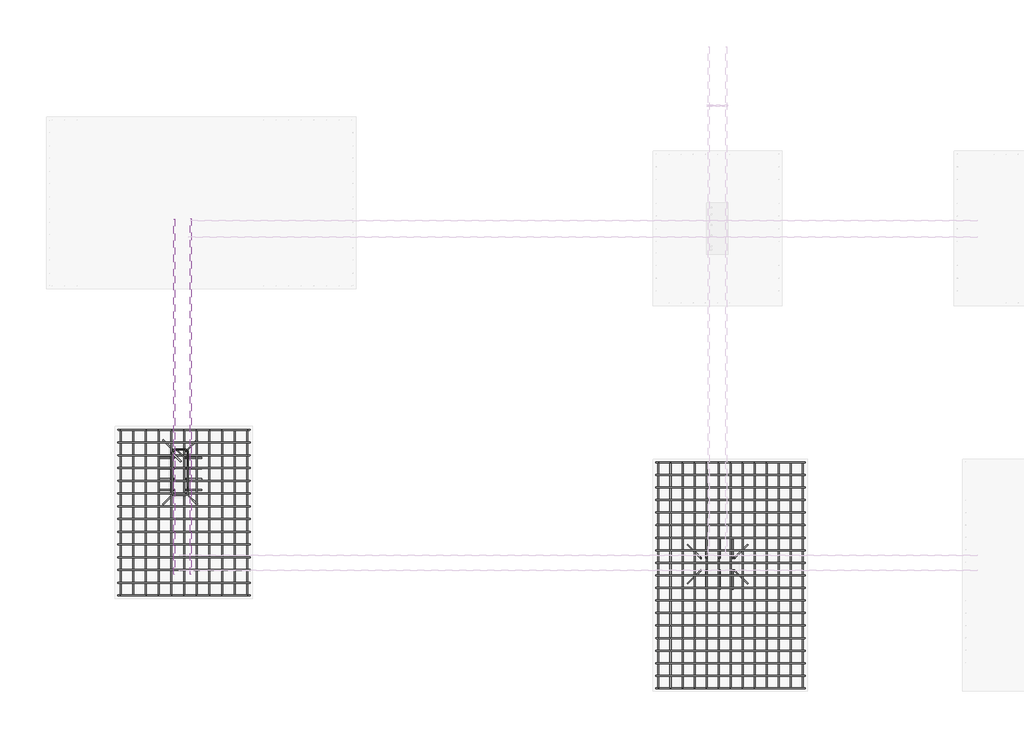
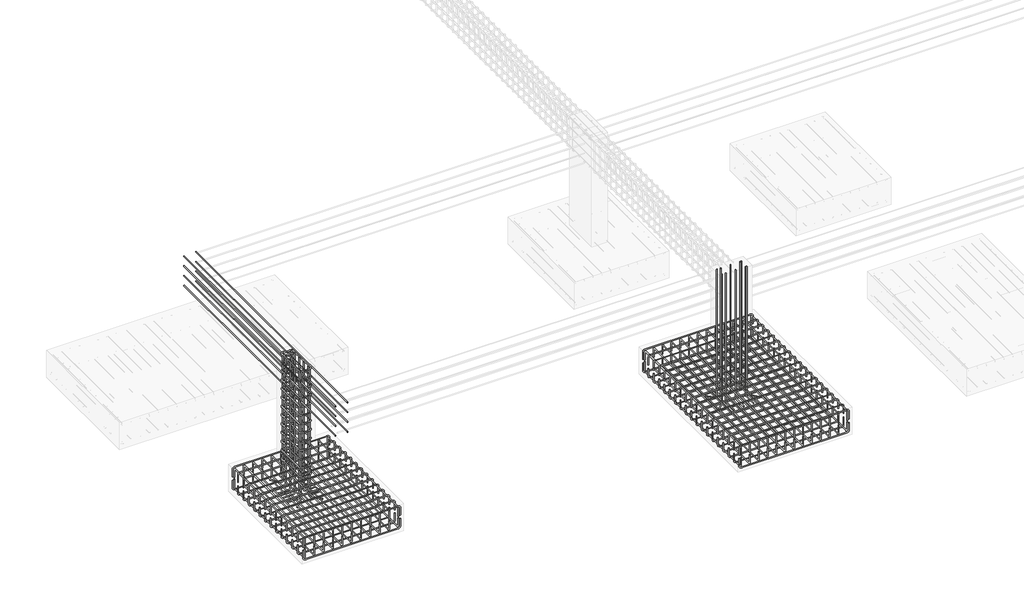
# One storey, part 2 of 16: 23 reinforcing bars.
"""IFC4 building model written with IfcOpenShell, lengths in millimetres."""

from ifc_helpers import new_model, si_unit, point, frame, origin, place, context, project, spatial, polyline, circle_curve, trimmed, segment, composite_curve, source, transform, mapped, element, save
from ifc_brep_helpers import swept_disk

model = new_model("IFC4")

# Units and contexts
model_context = context("Model", 3, world=origin())
ifc_project = project(units=[si_unit("LENGTHUNIT", "METRE", prefix="MILLI")], contexts=[model_context])

# Site, building, storey
site = spatial("IfcSite", under=ifc_project)
building = spatial("IfcBuilding", under=site)
storey = spatial("IfcBuildingStorey", under=building, Elevation=-1828.8)

# Reinforcing bars
placement = place(None, origin())
reinforcing_bar_shape = source(origin(), model_context, "Body", "SolidModel", [
    swept_disk(composite_curve([segment(polyline([(-7914.2725801, -5094.4085501, -2088.8), (-7914.2725801, -5094.4085501, -2212.8)]), True, "CONTINUOUS"), segment(trimmed(circle_curve(frame((-7944.2725801, -5094.4085501, -2212.8), z_axis=(0.0, 1.0, 0.0), x_axis=(30.0, 0.0, 0.0)), 30.0), [point((-7914.2725801, -5094.4085501, -2212.8))], [point((-7944.2725801, -5094.4085501, -2242.8))], True, "CARTESIAN"), True, "CONTINUOUS"), segment(polyline([(-7944.2725801, -5094.4085501, -2242.8), (-9612.2725801, -5094.4085501, -2242.8)]), True, "CONTINUOUS"), segment(trimmed(circle_curve(frame((-9612.2725801, -5094.4085501, -2212.8), z_axis=(0.0, 1.0, 0.0), x_axis=(0.0, 0.0, -30.0)), 30.0), [point((-9612.2725801, -5094.4085501, -2242.8))], [point((-9642.2725801, -5094.4085501, -2212.8))], True, "CARTESIAN"), True, "CONTINUOUS"), segment(polyline([(-9642.2725801, -5094.4085501, -2212.8), (-9642.2725801, -5094.4085501, -2088.8)]), True, "CONTINUOUS")], self_intersect=False), 6.0),
])
element("IfcReinforcingBar", 1, at=placement, inside=storey, context=model_context, shape_type="MappedRepresentation", body=[
    mapped(reinforcing_bar_shape, transform((0.0, 0.0, 0.0), x_axis=(1.0, 0.0, 0.0), y_axis=(0.0, 1.0, 0.0), z_axis=(0.0, 0.0, 1.0))),
    mapped(reinforcing_bar_shape, transform((0.0, -146.0, 0.0), x_axis=(1.0, 0.0, 0.0), y_axis=(0.0, 1.0, 0.0), z_axis=(0.0, 0.0, 1.0))),
    mapped(reinforcing_bar_shape, transform((0.0, -292.0, 0.0), x_axis=(1.0, 0.0, 0.0), y_axis=(0.0, 1.0, 0.0), z_axis=(0.0, 0.0, 1.0))),
    mapped(reinforcing_bar_shape, transform((0.0, -438.0, 0.0), x_axis=(1.0, 0.0, 0.0), y_axis=(0.0, 1.0, 0.0), z_axis=(0.0, 0.0, 1.0))),
    mapped(reinforcing_bar_shape, transform((0.0, -584.0, 0.0), x_axis=(1.0, 0.0, 0.0), y_axis=(0.0, 1.0, 0.0), z_axis=(0.0, 0.0, 1.0))),
    mapped(reinforcing_bar_shape, transform((0.0, -730.0, 0.0), x_axis=(1.0, 0.0, 0.0), y_axis=(0.0, 1.0, 0.0), z_axis=(0.0, 0.0, 1.0))),
    mapped(reinforcing_bar_shape, transform((0.0, -876.0, 0.0), x_axis=(1.0, 0.0, 0.0), y_axis=(0.0, 1.0, 0.0), z_axis=(0.0, 0.0, 1.0))),
    mapped(reinforcing_bar_shape, transform((0.0, -1022.0, 0.0), x_axis=(1.0, 0.0, 0.0), y_axis=(0.0, 1.0, 0.0), z_axis=(0.0, 0.0, 1.0))),
    mapped(reinforcing_bar_shape, transform((0.0, -1168.0, 0.0), x_axis=(1.0, 0.0, 0.0), y_axis=(0.0, 1.0, 0.0), z_axis=(0.0, 0.0, 1.0))),
    mapped(reinforcing_bar_shape, transform((0.0, -1314.0, 0.0), x_axis=(1.0, 0.0, 0.0), y_axis=(0.0, 1.0, 0.0), z_axis=(0.0, 0.0, 1.0))),
    mapped(reinforcing_bar_shape, transform((0.0, -1460.0, 0.0), x_axis=(1.0, 0.0, 0.0), y_axis=(0.0, 1.0, 0.0), z_axis=(0.0, 0.0, 1.0))),
    mapped(reinforcing_bar_shape, transform((0.0, -1606.0, 0.0), x_axis=(1.0, 0.0, 0.0), y_axis=(0.0, 1.0, 0.0), z_axis=(0.0, 0.0, 1.0))),
    mapped(reinforcing_bar_shape, transform((0.0, -1752.0, 0.0), x_axis=(1.0, 0.0, 0.0), y_axis=(0.0, 1.0, 0.0), z_axis=(0.0, 0.0, 1.0))),
    mapped(reinforcing_bar_shape, transform((0.0, -1898.0, 0.0), x_axis=(1.0, 0.0, 0.0), y_axis=(0.0, 1.0, 0.0), z_axis=(0.0, 0.0, 1.0))),
    mapped(reinforcing_bar_shape, transform((0.0, -2044.0, 0.0), x_axis=(1.0, 0.0, 0.0), y_axis=(0.0, 1.0, 0.0), z_axis=(0.0, 0.0, 1.0))),
    mapped(reinforcing_bar_shape, transform((0.0, -2190.0, 0.0), x_axis=(1.0, 0.0, 0.0), y_axis=(0.0, 1.0, 0.0), z_axis=(0.0, 0.0, 1.0))),
    mapped(reinforcing_bar_shape, transform((0.0, -2336.0, 0.0), x_axis=(1.0, 0.0, 0.0), y_axis=(0.0, 1.0, 0.0), z_axis=(0.0, 0.0, 1.0))),
    mapped(reinforcing_bar_shape, transform((0.0, -2482.0, 0.0), x_axis=(1.0, 0.0, 0.0), y_axis=(0.0, 1.0, 0.0), z_axis=(0.0, 0.0, 1.0))),
    mapped(reinforcing_bar_shape, transform((0.0, -2628.0, 0.0), x_axis=(1.0, 0.0, 0.0), y_axis=(0.0, 1.0, 0.0), z_axis=(0.0, 0.0, 1.0))),
])
reinforcing_bar_2_shape = source(origin(), model_context, "Body", "SolidModel", [
    swept_disk(composite_curve([segment(polyline([(-9642.2725801, -5094.4085501, -2024.671783), (-9642.2725801, -5094.4085501, -1900.671783)]), True, "CONTINUOUS"), segment(trimmed(circle_curve(frame((-9612.2725801, -5094.4085501, -1900.671783), z_axis=(0.0, 1.0, 0.0), x_axis=(-30.0, 0.0, 0.0)), 30.0), [point((-9642.2725801, -5094.4085501, -1900.671783))], [point((-9612.2725801, -5094.4085501, -1870.671783))], True, "CARTESIAN"), True, "CONTINUOUS"), segment(polyline([(-9612.2725801, -5094.4085501, -1870.671783), (-7944.2725801, -5094.4085501, -1870.671783)]), True, "CONTINUOUS"), segment(trimmed(circle_curve(frame((-7944.2725801, -5094.4085501, -1900.671783), z_axis=(0.0, 1.0, 0.0), x_axis=(0.0, 0.0, 30.0)), 30.0), [point((-7944.2725801, -5094.4085501, -1870.671783))], [point((-7914.2725801, -5094.4085501, -1900.671783))], True, "CARTESIAN"), True, "CONTINUOUS"), segment(polyline([(-7914.2725801, -5094.4085501, -1900.671783), (-7914.2725801, -5094.4085501, -2024.671783)]), True, "CONTINUOUS")], self_intersect=False), 6.0),
])
element("IfcReinforcingBar", 2, at=placement, inside=storey, context=model_context, shape_type="MappedRepresentation", body=[
    mapped(reinforcing_bar_2_shape, transform((0.0, 0.0, 0.0), x_axis=(1.0, 0.0, 0.0), y_axis=(0.0, 1.0, 0.0), z_axis=(0.0, 0.0, 1.0))),
    mapped(reinforcing_bar_2_shape, transform((0.0, -146.0, 0.0), x_axis=(1.0, 0.0, 0.0), y_axis=(0.0, 1.0, 0.0), z_axis=(0.0, 0.0, 1.0))),
    mapped(reinforcing_bar_2_shape, transform((0.0, -292.0, 0.0), x_axis=(1.0, 0.0, 0.0), y_axis=(0.0, 1.0, 0.0), z_axis=(0.0, 0.0, 1.0))),
    mapped(reinforcing_bar_2_shape, transform((0.0, -438.0, 0.0), x_axis=(1.0, 0.0, 0.0), y_axis=(0.0, 1.0, 0.0), z_axis=(0.0, 0.0, 1.0))),
    mapped(reinforcing_bar_2_shape, transform((0.0, -584.0, 0.0), x_axis=(1.0, 0.0, 0.0), y_axis=(0.0, 1.0, 0.0), z_axis=(0.0, 0.0, 1.0))),
    mapped(reinforcing_bar_2_shape, transform((0.0, -730.0, 0.0), x_axis=(1.0, 0.0, 0.0), y_axis=(0.0, 1.0, 0.0), z_axis=(0.0, 0.0, 1.0))),
    mapped(reinforcing_bar_2_shape, transform((0.0, -876.0, 0.0), x_axis=(1.0, 0.0, 0.0), y_axis=(0.0, 1.0, 0.0), z_axis=(0.0, 0.0, 1.0))),
    mapped(reinforcing_bar_2_shape, transform((0.0, -1022.0, 0.0), x_axis=(1.0, 0.0, 0.0), y_axis=(0.0, 1.0, 0.0), z_axis=(0.0, 0.0, 1.0))),
    mapped(reinforcing_bar_2_shape, transform((0.0, -1168.0, 0.0), x_axis=(1.0, 0.0, 0.0), y_axis=(0.0, 1.0, 0.0), z_axis=(0.0, 0.0, 1.0))),
    mapped(reinforcing_bar_2_shape, transform((0.0, -1314.0, 0.0), x_axis=(1.0, 0.0, 0.0), y_axis=(0.0, 1.0, 0.0), z_axis=(0.0, 0.0, 1.0))),
    mapped(reinforcing_bar_2_shape, transform((0.0, -1460.0, 0.0), x_axis=(1.0, 0.0, 0.0), y_axis=(0.0, 1.0, 0.0), z_axis=(0.0, 0.0, 1.0))),
    mapped(reinforcing_bar_2_shape, transform((0.0, -1606.0, 0.0), x_axis=(1.0, 0.0, 0.0), y_axis=(0.0, 1.0, 0.0), z_axis=(0.0, 0.0, 1.0))),
    mapped(reinforcing_bar_2_shape, transform((0.0, -1752.0, 0.0), x_axis=(1.0, 0.0, 0.0), y_axis=(0.0, 1.0, 0.0), z_axis=(0.0, 0.0, 1.0))),
    mapped(reinforcing_bar_2_shape, transform((0.0, -1898.0, 0.0), x_axis=(1.0, 0.0, 0.0), y_axis=(0.0, 1.0, 0.0), z_axis=(0.0, 0.0, 1.0))),
    mapped(reinforcing_bar_2_shape, transform((0.0, -2044.0, 0.0), x_axis=(1.0, 0.0, 0.0), y_axis=(0.0, 1.0, 0.0), z_axis=(0.0, 0.0, 1.0))),
    mapped(reinforcing_bar_2_shape, transform((0.0, -2190.0, 0.0), x_axis=(1.0, 0.0, 0.0), y_axis=(0.0, 1.0, 0.0), z_axis=(0.0, 0.0, 1.0))),
    mapped(reinforcing_bar_2_shape, transform((0.0, -2336.0, 0.0), x_axis=(1.0, 0.0, 0.0), y_axis=(0.0, 1.0, 0.0), z_axis=(0.0, 0.0, 1.0))),
    mapped(reinforcing_bar_2_shape, transform((0.0, -2482.0, 0.0), x_axis=(1.0, 0.0, 0.0), y_axis=(0.0, 1.0, 0.0), z_axis=(0.0, 0.0, 1.0))),
    mapped(reinforcing_bar_2_shape, transform((0.0, -2628.0, 0.0), x_axis=(1.0, 0.0, 0.0), y_axis=(0.0, 1.0, 0.0), z_axis=(0.0, 0.0, 1.0))),
])
reinforcing_bar_3_shape = source(origin(), model_context, "Body", "SolidModel", [
    swept_disk(composite_curve([segment(polyline([(-9615.8984804, -5094.4085501, -2074.8303715), (-9615.8984804, -5094.4085501, -2198.8303715)]), True, "CONTINUOUS"), segment(trimmed(circle_curve(frame((-9615.8984804, -5124.4085501, -2198.8303715), z_axis=(-1.0, 0.0, 0.0), x_axis=(0.0, 30.0, 0.0)), 30.0), [point((-9615.8984804, -5094.4085501, -2198.8303715))], [point((-9615.8984804, -5124.4085501, -2228.8303715))], True, "CARTESIAN"), True, "CONTINUOUS"), segment(polyline([(-9615.8984804, -5124.4085501, -2228.8303715), (-9615.8984804, -7692.4085501, -2228.8303715)]), True, "CONTINUOUS"), segment(trimmed(circle_curve(frame((-9615.8984804, -7692.4085501, -2198.8303715), z_axis=(-1.0, 0.0, 0.0), x_axis=(0.0, 0.0, -30.0)), 30.0), [point((-9615.8984804, -7692.4085501, -2228.8303715))], [point((-9615.8984804, -7722.4085501, -2198.8303715))], True, "CARTESIAN"), True, "CONTINUOUS"), segment(polyline([(-9615.8984804, -7722.4085501, -2198.8303715), (-9615.8984804, -7722.4085501, -2074.8303715)]), True, "CONTINUOUS")], self_intersect=False), 6.0),
])
element("IfcReinforcingBar", 3, at=placement, inside=storey, context=model_context, shape_type="MappedRepresentation", body=[
    mapped(reinforcing_bar_3_shape, transform((0.0, 0.0, 0.0), x_axis=(1.0, 0.0, 0.0), y_axis=(0.0, 1.0, 0.0), z_axis=(0.0, 0.0, 1.0))),
    mapped(reinforcing_bar_3_shape, transform((139.7704391, 0.0, 0.0), x_axis=(1.0, 0.0, 0.0), y_axis=(0.0, 1.0, 0.0), z_axis=(0.0, 0.0, 1.0))),
    mapped(reinforcing_bar_3_shape, transform((279.5408781, 0.0, 0.0), x_axis=(1.0, 0.0, 0.0), y_axis=(0.0, 1.0, 0.0), z_axis=(0.0, 0.0, 1.0))),
    mapped(reinforcing_bar_3_shape, transform((419.3113172, 0.0, 0.0), x_axis=(1.0, 0.0, 0.0), y_axis=(0.0, 1.0, 0.0), z_axis=(0.0, 0.0, 1.0))),
    mapped(reinforcing_bar_3_shape, transform((559.0817562, 0.0, 0.0), x_axis=(1.0, 0.0, 0.0), y_axis=(0.0, 1.0, 0.0), z_axis=(0.0, 0.0, 1.0))),
    mapped(reinforcing_bar_3_shape, transform((698.8521953, 0.0, 0.0), x_axis=(1.0, 0.0, 0.0), y_axis=(0.0, 1.0, 0.0), z_axis=(0.0, 0.0, 1.0))),
    mapped(reinforcing_bar_3_shape, transform((838.6226343, 0.0, 0.0), x_axis=(1.0, 0.0, 0.0), y_axis=(0.0, 1.0, 0.0), z_axis=(0.0, 0.0, 1.0))),
    mapped(reinforcing_bar_3_shape, transform((978.3930734, 0.0, 0.0), x_axis=(1.0, 0.0, 0.0), y_axis=(0.0, 1.0, 0.0), z_axis=(0.0, 0.0, 1.0))),
    mapped(reinforcing_bar_3_shape, transform((1118.1635125, 0.0, 0.0), x_axis=(1.0, 0.0, 0.0), y_axis=(0.0, 1.0, 0.0), z_axis=(0.0, 0.0, 1.0))),
    mapped(reinforcing_bar_3_shape, transform((1257.9339515, 0.0, 0.0), x_axis=(1.0, 0.0, 0.0), y_axis=(0.0, 1.0, 0.0), z_axis=(0.0, 0.0, 1.0))),
    mapped(reinforcing_bar_3_shape, transform((1397.7043906, 0.0, 0.0), x_axis=(1.0, 0.0, 0.0), y_axis=(0.0, 1.0, 0.0), z_axis=(0.0, 0.0, 1.0))),
    mapped(reinforcing_bar_3_shape, transform((1537.4748296, 0.0, 0.0), x_axis=(1.0, 0.0, 0.0), y_axis=(0.0, 1.0, 0.0), z_axis=(0.0, 0.0, 1.0))),
    mapped(reinforcing_bar_3_shape, transform((1677.2452687, 0.0, 0.0), x_axis=(1.0, 0.0, 0.0), y_axis=(0.0, 1.0, 0.0), z_axis=(0.0, 0.0, 1.0))),
])
reinforcing_bar_4_shape = source(origin(), model_context, "Body", "SolidModel", [
    swept_disk(composite_curve([segment(polyline([(-7938.6532117, -5094.4085501, -2038.9453456), (-7938.6532117, -5094.4085501, -1914.9453456)]), True, "CONTINUOUS"), segment(trimmed(circle_curve(frame((-7938.6532117, -5124.4085501, -1914.9453456), z_axis=(1.0, 0.0, 0.0), x_axis=(0.0, 30.0, 0.0)), 30.0), [point((-7938.6532117, -5094.4085501, -1914.9453456))], [point((-7938.6532117, -5124.4085501, -1884.9453456))], True, "CARTESIAN"), True, "CONTINUOUS"), segment(polyline([(-7938.6532117, -5124.4085501, -1884.9453456), (-7938.6532117, -7692.4085501, -1884.9453456)]), True, "CONTINUOUS"), segment(trimmed(circle_curve(frame((-7938.6532117, -7692.4085501, -1914.9453456), z_axis=(1.0, 0.0, 0.0), x_axis=(0.0, 0.0, 30.0)), 30.0), [point((-7938.6532117, -7692.4085501, -1884.9453456))], [point((-7938.6532117, -7722.4085501, -1914.9453456))], True, "CARTESIAN"), True, "CONTINUOUS"), segment(polyline([(-7938.6532117, -7722.4085501, -1914.9453456), (-7938.6532117, -7722.4085501, -2038.9453456)]), True, "CONTINUOUS")], self_intersect=False), 6.0),
])
element("IfcReinforcingBar", 4, at=placement, inside=storey, context=model_context, shape_type="MappedRepresentation", body=[
    mapped(reinforcing_bar_4_shape, transform((0.0, 0.0, 0.0), x_axis=(1.0, 0.0, 0.0), y_axis=(0.0, 1.0, 0.0), z_axis=(0.0, 0.0, 1.0))),
    mapped(reinforcing_bar_4_shape, transform((-139.7704391, 0.0, 0.0), x_axis=(1.0, 0.0, 0.0), y_axis=(0.0, 1.0, 0.0), z_axis=(0.0, 0.0, 1.0))),
    mapped(reinforcing_bar_4_shape, transform((-279.5408781, 0.0, 0.0), x_axis=(1.0, 0.0, 0.0), y_axis=(0.0, 1.0, 0.0), z_axis=(0.0, 0.0, 1.0))),
    mapped(reinforcing_bar_4_shape, transform((-419.3113172, 0.0, 0.0), x_axis=(1.0, 0.0, 0.0), y_axis=(0.0, 1.0, 0.0), z_axis=(0.0, 0.0, 1.0))),
    mapped(reinforcing_bar_4_shape, transform((-559.0817562, 0.0, 0.0), x_axis=(1.0, 0.0, 0.0), y_axis=(0.0, 1.0, 0.0), z_axis=(0.0, 0.0, 1.0))),
    mapped(reinforcing_bar_4_shape, transform((-698.8521953, 0.0, 0.0), x_axis=(1.0, 0.0, 0.0), y_axis=(0.0, 1.0, 0.0), z_axis=(0.0, 0.0, 1.0))),
    mapped(reinforcing_bar_4_shape, transform((-838.6226343, 0.0, 0.0), x_axis=(1.0, 0.0, 0.0), y_axis=(0.0, 1.0, 0.0), z_axis=(0.0, 0.0, 1.0))),
    mapped(reinforcing_bar_4_shape, transform((-978.3930734, 0.0, 0.0), x_axis=(1.0, 0.0, 0.0), y_axis=(0.0, 1.0, 0.0), z_axis=(0.0, 0.0, 1.0))),
    mapped(reinforcing_bar_4_shape, transform((-1118.1635125, 0.0, 0.0), x_axis=(1.0, 0.0, 0.0), y_axis=(0.0, 1.0, 0.0), z_axis=(0.0, 0.0, 1.0))),
    mapped(reinforcing_bar_4_shape, transform((-1257.9339515, 0.0, 0.0), x_axis=(1.0, 0.0, 0.0), y_axis=(0.0, 1.0, 0.0), z_axis=(0.0, 0.0, 1.0))),
    mapped(reinforcing_bar_4_shape, transform((-1397.7043906, 0.0, 0.0), x_axis=(1.0, 0.0, 0.0), y_axis=(0.0, 1.0, 0.0), z_axis=(0.0, 0.0, 1.0))),
    mapped(reinforcing_bar_4_shape, transform((-1537.4748296, 0.0, 0.0), x_axis=(1.0, 0.0, 0.0), y_axis=(0.0, 1.0, 0.0), z_axis=(0.0, 0.0, 1.0))),
    mapped(reinforcing_bar_4_shape, transform((-1677.2452687, 0.0, 0.0), x_axis=(1.0, 0.0, 0.0), y_axis=(0.0, 1.0, 0.0), z_axis=(0.0, 0.0, 1.0))),
])
reinforcing_bar_5_shape = source(origin(), model_context, "Body", "SolidModel", [
    swept_disk(composite_curve([segment(polyline([(-14366.5528212, -4715.1308991, -2085.9710757), (-14366.5528212, -4715.1308991, -2209.9710757)]), True, "CONTINUOUS"), segment(trimmed(circle_curve(frame((-14396.5528212, -4715.1308991, -2209.9710757), z_axis=(0.0, 1.0, 0.0), x_axis=(30.0, 0.0, 0.0)), 30.0), [point((-14366.5528212, -4715.1308991, -2209.9710757))], [point((-14396.5528212, -4715.1308991, -2239.9710757))], True, "CARTESIAN"), True, "CONTINUOUS"), segment(polyline([(-14396.5528212, -4715.1308991, -2239.9710757), (-15864.5528212, -4715.1308991, -2239.9710757)]), True, "CONTINUOUS"), segment(trimmed(circle_curve(frame((-15864.5528212, -4715.1308991, -2209.9710757), z_axis=(0.0, 1.0, 0.0), x_axis=(0.0, 0.0, -30.0)), 30.0), [point((-15864.5528212, -4715.1308991, -2239.9710757))], [point((-15894.5528212, -4715.1308991, -2209.9710757))], True, "CARTESIAN"), True, "CONTINUOUS"), segment(polyline([(-15894.5528212, -4715.1308991, -2209.9710757), (-15894.5528212, -4715.1308991, -2085.9710757)]), True, "CONTINUOUS")], self_intersect=False), 6.0),
])
element("IfcReinforcingBar", 5, at=placement, inside=storey, context=model_context, shape_type="MappedRepresentation", body=[
    mapped(reinforcing_bar_5_shape, transform((0.0, 0.0, 0.0), x_axis=(1.0, 0.0, 0.0), y_axis=(0.0, 1.0, 0.0), z_axis=(0.0, 0.0, 1.0))),
    mapped(reinforcing_bar_5_shape, transform((0.0, -148.3076923, 0.0), x_axis=(1.0, 0.0, 0.0), y_axis=(0.0, 1.0, 0.0), z_axis=(0.0, 0.0, 1.0))),
    mapped(reinforcing_bar_5_shape, transform((0.0, -296.6153846, 0.0), x_axis=(1.0, 0.0, 0.0), y_axis=(0.0, 1.0, 0.0), z_axis=(0.0, 0.0, 1.0))),
    mapped(reinforcing_bar_5_shape, transform((0.0, -444.9230769, 0.0), x_axis=(1.0, 0.0, 0.0), y_axis=(0.0, 1.0, 0.0), z_axis=(0.0, 0.0, 1.0))),
    mapped(reinforcing_bar_5_shape, transform((0.0, -593.2307692, 0.0), x_axis=(1.0, 0.0, 0.0), y_axis=(0.0, 1.0, 0.0), z_axis=(0.0, 0.0, 1.0))),
    mapped(reinforcing_bar_5_shape, transform((0.0, -741.5384615, 0.0), x_axis=(1.0, 0.0, 0.0), y_axis=(0.0, 1.0, 0.0), z_axis=(0.0, 0.0, 1.0))),
    mapped(reinforcing_bar_5_shape, transform((0.0, -889.8461538, 0.0), x_axis=(1.0, 0.0, 0.0), y_axis=(0.0, 1.0, 0.0), z_axis=(0.0, 0.0, 1.0))),
    mapped(reinforcing_bar_5_shape, transform((0.0, -1038.1538462, 0.0), x_axis=(1.0, 0.0, 0.0), y_axis=(0.0, 1.0, 0.0), z_axis=(0.0, 0.0, 1.0))),
    mapped(reinforcing_bar_5_shape, transform((0.0, -1186.4615385, 0.0), x_axis=(1.0, 0.0, 0.0), y_axis=(0.0, 1.0, 0.0), z_axis=(0.0, 0.0, 1.0))),
    mapped(reinforcing_bar_5_shape, transform((0.0, -1334.7692308, 0.0), x_axis=(1.0, 0.0, 0.0), y_axis=(0.0, 1.0, 0.0), z_axis=(0.0, 0.0, 1.0))),
    mapped(reinforcing_bar_5_shape, transform((0.0, -1483.0769231, 0.0), x_axis=(1.0, 0.0, 0.0), y_axis=(0.0, 1.0, 0.0), z_axis=(0.0, 0.0, 1.0))),
    mapped(reinforcing_bar_5_shape, transform((0.0, -1631.3846154, 0.0), x_axis=(1.0, 0.0, 0.0), y_axis=(0.0, 1.0, 0.0), z_axis=(0.0, 0.0, 1.0))),
    mapped(reinforcing_bar_5_shape, transform((0.0, -1779.6923077, 0.0), x_axis=(1.0, 0.0, 0.0), y_axis=(0.0, 1.0, 0.0), z_axis=(0.0, 0.0, 1.0))),
    mapped(reinforcing_bar_5_shape, transform((0.0, -1928.0, 0.0), x_axis=(1.0, 0.0, 0.0), y_axis=(0.0, 1.0, 0.0), z_axis=(0.0, 0.0, 1.0))),
])
reinforcing_bar_6_shape = source(origin(), model_context, "Body", "SolidModel", [
    swept_disk(composite_curve([segment(polyline([(-15894.5528212, -4715.1308991, -2024.6601121), (-15894.5528212, -4715.1308991, -1900.6601121)]), True, "CONTINUOUS"), segment(trimmed(circle_curve(frame((-15864.5528212, -4715.1308991, -1900.6601121), z_axis=(0.0, 1.0, 0.0), x_axis=(-30.0, 0.0, 0.0)), 30.0), [point((-15894.5528212, -4715.1308991, -1900.6601121))], [point((-15864.5528212, -4715.1308991, -1870.6601121))], True, "CARTESIAN"), True, "CONTINUOUS"), segment(polyline([(-15864.5528212, -4715.1308991, -1870.6601121), (-14396.5528212, -4715.1308991, -1870.6601121)]), True, "CONTINUOUS"), segment(trimmed(circle_curve(frame((-14396.5528212, -4715.1308991, -1900.6601121), z_axis=(0.0, 1.0, 0.0), x_axis=(0.0, 0.0, 30.0)), 30.0), [point((-14396.5528212, -4715.1308991, -1870.6601121))], [point((-14366.5528212, -4715.1308991, -1900.6601121))], True, "CARTESIAN"), True, "CONTINUOUS"), segment(polyline([(-14366.5528212, -4715.1308991, -1900.6601121), (-14366.5528212, -4715.1308991, -2024.6601121)]), True, "CONTINUOUS")], self_intersect=False), 6.0),
])
element("IfcReinforcingBar", 6, at=placement, inside=storey, context=model_context, shape_type="MappedRepresentation", body=[
    mapped(reinforcing_bar_6_shape, transform((0.0, 0.0, 0.0), x_axis=(1.0, 0.0, 0.0), y_axis=(0.0, 1.0, 0.0), z_axis=(0.0, 0.0, 1.0))),
    mapped(reinforcing_bar_6_shape, transform((0.0, -148.3076923, 0.0), x_axis=(1.0, 0.0, 0.0), y_axis=(0.0, 1.0, 0.0), z_axis=(0.0, 0.0, 1.0))),
    mapped(reinforcing_bar_6_shape, transform((0.0, -296.6153846, 0.0), x_axis=(1.0, 0.0, 0.0), y_axis=(0.0, 1.0, 0.0), z_axis=(0.0, 0.0, 1.0))),
    mapped(reinforcing_bar_6_shape, transform((0.0, -444.9230769, 0.0), x_axis=(1.0, 0.0, 0.0), y_axis=(0.0, 1.0, 0.0), z_axis=(0.0, 0.0, 1.0))),
    mapped(reinforcing_bar_6_shape, transform((0.0, -593.2307692, 0.0), x_axis=(1.0, 0.0, 0.0), y_axis=(0.0, 1.0, 0.0), z_axis=(0.0, 0.0, 1.0))),
    mapped(reinforcing_bar_6_shape, transform((0.0, -741.5384615, 0.0), x_axis=(1.0, 0.0, 0.0), y_axis=(0.0, 1.0, 0.0), z_axis=(0.0, 0.0, 1.0))),
    mapped(reinforcing_bar_6_shape, transform((0.0, -889.8461538, 0.0), x_axis=(1.0, 0.0, 0.0), y_axis=(0.0, 1.0, 0.0), z_axis=(0.0, 0.0, 1.0))),
    mapped(reinforcing_bar_6_shape, transform((0.0, -1038.1538462, 0.0), x_axis=(1.0, 0.0, 0.0), y_axis=(0.0, 1.0, 0.0), z_axis=(0.0, 0.0, 1.0))),
    mapped(reinforcing_bar_6_shape, transform((0.0, -1186.4615385, 0.0), x_axis=(1.0, 0.0, 0.0), y_axis=(0.0, 1.0, 0.0), z_axis=(0.0, 0.0, 1.0))),
    mapped(reinforcing_bar_6_shape, transform((0.0, -1334.7692308, 0.0), x_axis=(1.0, 0.0, 0.0), y_axis=(0.0, 1.0, 0.0), z_axis=(0.0, 0.0, 1.0))),
    mapped(reinforcing_bar_6_shape, transform((0.0, -1483.0769231, 0.0), x_axis=(1.0, 0.0, 0.0), y_axis=(0.0, 1.0, 0.0), z_axis=(0.0, 0.0, 1.0))),
    mapped(reinforcing_bar_6_shape, transform((0.0, -1631.3846154, 0.0), x_axis=(1.0, 0.0, 0.0), y_axis=(0.0, 1.0, 0.0), z_axis=(0.0, 0.0, 1.0))),
    mapped(reinforcing_bar_6_shape, transform((0.0, -1779.6923077, 0.0), x_axis=(1.0, 0.0, 0.0), y_axis=(0.0, 1.0, 0.0), z_axis=(0.0, 0.0, 1.0))),
    mapped(reinforcing_bar_6_shape, transform((0.0, -1928.0, 0.0), x_axis=(1.0, 0.0, 0.0), y_axis=(0.0, 1.0, 0.0), z_axis=(0.0, 0.0, 1.0))),
])
reinforcing_bar_7_shape = source(origin(), model_context, "Body", "SolidModel", [
    swept_disk(composite_curve([segment(polyline([(-15867.8311901, -4715.1308991, -2068.2398219), (-15867.8311901, -4715.1308991, -2192.2398219)]), True, "CONTINUOUS"), segment(trimmed(circle_curve(frame((-15867.8311901, -4745.1308991, -2192.2398219), z_axis=(-1.0, 0.0, 0.0), x_axis=(0.0, 30.0, 0.0)), 30.0), [point((-15867.8311901, -4715.1308991, -2192.2398219))], [point((-15867.8311901, -4745.1308991, -2222.2398219))], True, "CARTESIAN"), True, "CONTINUOUS"), segment(polyline([(-15867.8311901, -4745.1308991, -2222.2398219), (-15867.8311901, -6613.1308991, -2222.2398219)]), True, "CONTINUOUS"), segment(trimmed(circle_curve(frame((-15867.8311901, -6613.1308991, -2192.2398219), z_axis=(-1.0, 0.0, 0.0), x_axis=(0.0, 0.0, -30.0)), 30.0), [point((-15867.8311901, -6613.1308991, -2222.2398219))], [point((-15867.8311901, -6643.1308991, -2192.2398219))], True, "CARTESIAN"), True, "CONTINUOUS"), segment(polyline([(-15867.8311901, -6643.1308991, -2192.2398219), (-15867.8311901, -6643.1308991, -2068.2398219)]), True, "CONTINUOUS")], self_intersect=False), 6.0),
])
element("IfcReinforcingBar", 7, at=placement, inside=storey, context=model_context, shape_type="MappedRepresentation", body=[
    mapped(reinforcing_bar_7_shape, transform((0.0, 0.0, 0.0), x_axis=(1.0, 0.0, 0.0), y_axis=(0.0, 1.0, 0.0), z_axis=(0.0, 0.0, 1.0))),
    mapped(reinforcing_bar_7_shape, transform((147.4799613, 0.0, 0.0), x_axis=(1.0, 0.0, 0.0), y_axis=(0.0, 1.0, 0.0), z_axis=(0.0, 0.0, 1.0))),
    mapped(reinforcing_bar_7_shape, transform((294.9599226, 0.0, 0.0), x_axis=(1.0, 0.0, 0.0), y_axis=(0.0, 1.0, 0.0), z_axis=(0.0, 0.0, 1.0))),
    mapped(reinforcing_bar_7_shape, transform((442.4398839, 0.0, 0.0), x_axis=(1.0, 0.0, 0.0), y_axis=(0.0, 1.0, 0.0), z_axis=(0.0, 0.0, 1.0))),
    mapped(reinforcing_bar_7_shape, transform((589.9198452, 0.0, 0.0), x_axis=(1.0, 0.0, 0.0), y_axis=(0.0, 1.0, 0.0), z_axis=(0.0, 0.0, 1.0))),
    mapped(reinforcing_bar_7_shape, transform((737.3998065, 0.0, 0.0), x_axis=(1.0, 0.0, 0.0), y_axis=(0.0, 1.0, 0.0), z_axis=(0.0, 0.0, 1.0))),
    mapped(reinforcing_bar_7_shape, transform((884.8797678, 0.0, 0.0), x_axis=(1.0, 0.0, 0.0), y_axis=(0.0, 1.0, 0.0), z_axis=(0.0, 0.0, 1.0))),
    mapped(reinforcing_bar_7_shape, transform((1032.359729, 0.0, 0.0), x_axis=(1.0, 0.0, 0.0), y_axis=(0.0, 1.0, 0.0), z_axis=(0.0, 0.0, 1.0))),
    mapped(reinforcing_bar_7_shape, transform((1179.8396903, 0.0, 0.0), x_axis=(1.0, 0.0, 0.0), y_axis=(0.0, 1.0, 0.0), z_axis=(0.0, 0.0, 1.0))),
    mapped(reinforcing_bar_7_shape, transform((1327.3196516, 0.0, 0.0), x_axis=(1.0, 0.0, 0.0), y_axis=(0.0, 1.0, 0.0), z_axis=(0.0, 0.0, 1.0))),
    mapped(reinforcing_bar_7_shape, transform((1474.7996129, 0.0, 0.0), x_axis=(1.0, 0.0, 0.0), y_axis=(0.0, 1.0, 0.0), z_axis=(0.0, 0.0, 1.0))),
])
reinforcing_bar_8_shape = source(origin(), model_context, "Body", "SolidModel", [
    swept_disk(composite_curve([segment(polyline([(-14393.0315771, -4715.1308991, -2039.8547961), (-14393.0315771, -4715.1308991, -1915.8547961)]), True, "CONTINUOUS"), segment(trimmed(circle_curve(frame((-14393.0315771, -4745.1308991, -1915.8547961), z_axis=(1.0, 0.0, 0.0), x_axis=(0.0, 30.0, 0.0)), 30.0), [point((-14393.0315771, -4715.1308991, -1915.8547961))], [point((-14393.0315771, -4745.1308991, -1885.8547961))], True, "CARTESIAN"), True, "CONTINUOUS"), segment(polyline([(-14393.0315771, -4745.1308991, -1885.8547961), (-14393.0315771, -6613.1308991, -1885.8547961)]), True, "CONTINUOUS"), segment(trimmed(circle_curve(frame((-14393.0315771, -6613.1308991, -1915.8547961), z_axis=(1.0, 0.0, 0.0), x_axis=(0.0, 0.0, 30.0)), 30.0), [point((-14393.0315771, -6613.1308991, -1885.8547961))], [point((-14393.0315771, -6643.1308991, -1915.8547961))], True, "CARTESIAN"), True, "CONTINUOUS"), segment(polyline([(-14393.0315771, -6643.1308991, -1915.8547961), (-14393.0315771, -6643.1308991, -2039.8547961)]), True, "CONTINUOUS")], self_intersect=False), 6.0),
])
element("IfcReinforcingBar", 8, at=placement, inside=storey, context=model_context, shape_type="MappedRepresentation", body=[
    mapped(reinforcing_bar_8_shape, transform((0.0, 0.0, 0.0), x_axis=(1.0, 0.0, 0.0), y_axis=(0.0, 1.0, 0.0), z_axis=(0.0, 0.0, 1.0))),
    mapped(reinforcing_bar_8_shape, transform((-147.4799613, 0.0, 0.0), x_axis=(1.0, 0.0, 0.0), y_axis=(0.0, 1.0, 0.0), z_axis=(0.0, 0.0, 1.0))),
    mapped(reinforcing_bar_8_shape, transform((-294.9599226, 0.0, 0.0), x_axis=(1.0, 0.0, 0.0), y_axis=(0.0, 1.0, 0.0), z_axis=(0.0, 0.0, 1.0))),
    mapped(reinforcing_bar_8_shape, transform((-442.4398839, 0.0, 0.0), x_axis=(1.0, 0.0, 0.0), y_axis=(0.0, 1.0, 0.0), z_axis=(0.0, 0.0, 1.0))),
    mapped(reinforcing_bar_8_shape, transform((-589.9198452, 0.0, 0.0), x_axis=(1.0, 0.0, 0.0), y_axis=(0.0, 1.0, 0.0), z_axis=(0.0, 0.0, 1.0))),
    mapped(reinforcing_bar_8_shape, transform((-737.3998065, 0.0, 0.0), x_axis=(1.0, 0.0, 0.0), y_axis=(0.0, 1.0, 0.0), z_axis=(0.0, 0.0, 1.0))),
    mapped(reinforcing_bar_8_shape, transform((-884.8797678, 0.0, 0.0), x_axis=(1.0, 0.0, 0.0), y_axis=(0.0, 1.0, 0.0), z_axis=(0.0, 0.0, 1.0))),
    mapped(reinforcing_bar_8_shape, transform((-1032.359729, 0.0, 0.0), x_axis=(1.0, 0.0, 0.0), y_axis=(0.0, 1.0, 0.0), z_axis=(0.0, 0.0, 1.0))),
    mapped(reinforcing_bar_8_shape, transform((-1179.8396903, 0.0, 0.0), x_axis=(1.0, 0.0, 0.0), y_axis=(0.0, 1.0, 0.0), z_axis=(0.0, 0.0, 1.0))),
    mapped(reinforcing_bar_8_shape, transform((-1327.3196516, 0.0, 0.0), x_axis=(1.0, 0.0, 0.0), y_axis=(0.0, 1.0, 0.0), z_axis=(0.0, 0.0, 1.0))),
    mapped(reinforcing_bar_8_shape, transform((-1474.7996129, 0.0, 0.0), x_axis=(1.0, 0.0, 0.0), y_axis=(0.0, 1.0, 0.0), z_axis=(0.0, 0.0, 1.0))),
])
reinforcing_bar_9_shape = source(origin(), model_context, "Body", "SolidModel", [
    swept_disk(composite_curve([segment(polyline([(-9060.102427, -6208.8808991, -30.0), (-9060.102427, -6208.8808991, -2141.7459972)]), True, "CONTINUOUS"), segment(trimmed(circle_curve(frame((-9060.102427, -6178.8808991, -2141.7459972), z_axis=(1.0, 0.0, 0.0), x_axis=(0.0, -30.0, 0.0)), 30.0), [point((-9060.102427, -6208.8808991, -2141.7459972))], [point((-9060.102427, -6178.8808991, -2171.7459972))], True, "CARTESIAN"), True, "CONTINUOUS"), segment(polyline([(-9060.102427, -6178.8808991, -2171.7459972), (-9060.102427, -5988.2528007, -2171.7459972)]), True, "CONTINUOUS")], self_intersect=False), 6.0),
])
element("IfcReinforcingBar", 9, at=placement, inside=storey, context=model_context, shape_type="MappedRepresentation", body=[
    mapped(reinforcing_bar_9_shape, transform((0.0, 0.0, 0.0), x_axis=(1.0, 0.0, 0.0), y_axis=(0.0, 1.0, 0.0), z_axis=(0.0, 0.0, 1.0))),
    mapped(reinforcing_bar_9_shape, transform((153.9273626, 0.0, 0.0), x_axis=(1.0, 0.0, 0.0), y_axis=(0.0, 1.0, 0.0), z_axis=(0.0, 0.0, 1.0))),
    mapped(reinforcing_bar_9_shape, transform((307.8547253, 0.0, 0.0), x_axis=(1.0, 0.0, 0.0), y_axis=(0.0, 1.0, 0.0), z_axis=(0.0, 0.0, 1.0))),
])
element("IfcReinforcingBar", 10, at=placement, inside=storey, context=model_context, shape_type="SolidModel", body=[
    swept_disk(composite_curve([segment(polyline([(-9121.7720578, -6208.8808991, -30.0), (-9121.7720578, -6208.8808991, -2141.7459972)]), True, "CONTINUOUS"), segment(trimmed(circle_curve(frame((-9142.9852612, -6187.6676957, -2141.7459972), z_axis=(0.7071067811865477, 0.7071067811865474, 0.0), x_axis=(21.213203399998747, -21.213203399999657, 0.0)), 30.0), [point((-9121.7720578, -6208.8808991, -2141.7459972))], [point((-9142.9852612, -6187.6676957, -2171.7459972))], True, "CARTESIAN"), True, "CONTINUOUS"), segment(polyline([(-9142.9852612, -6187.6676957, -2171.7459972), (-9277.7796823, -6052.8732746, -2171.7459972)]), True, "CONTINUOUS")], self_intersect=False), 6.0),
])
element("IfcReinforcingBar", 11, at=placement, inside=storey, context=model_context, shape_type="SolidModel", body=[
    swept_disk(composite_curve([segment(polyline([(-9121.7720578, -6349.3808991, -30.0), (-9121.7720578, -6349.3808991, -2141.7459972)]), True, "CONTINUOUS"), segment(trimmed(circle_curve(frame((-9142.9852612, -6370.5941026, -2141.7459972), z_axis=(-0.7071067811865445, 0.7071067811865506, 0.0), x_axis=(21.213203399998747, 21.213203500000418, 0.0)), 30.0), [point((-9121.7720578, -6349.3808991, -2141.7459972))], [point((-9142.9852612, -6370.5941026, -2171.7459972))], True, "CARTESIAN"), True, "CONTINUOUS"), segment(polyline([(-9142.9852612, -6370.5941026, -2171.7459972), (-9277.7796823, -6505.3885237, -2171.7459972)]), True, "CONTINUOUS")], self_intersect=False), 6.0),
])
element("IfcReinforcingBar", 12, at=placement, inside=storey, context=model_context, shape_type="SolidModel", body=[
    swept_disk(composite_curve([segment(polyline([(-8734.7731024, -6349.3808991, -30.0), (-8734.7731024, -6349.3808991, -2141.7459972)]), True, "CONTINUOUS"), segment(trimmed(circle_curve(frame((-8713.559899, -6370.5941026, -2141.7459972), z_axis=(-0.7071067811865445, -0.7071067811865506, 0.0), x_axis=(-21.213203400000566, 21.213203500000418, 0.0)), 30.0), [point((-8734.7731024, -6349.3808991, -2141.7459972))], [point((-8713.559899, -6370.5941026, -2171.7459972))], True, "CARTESIAN"), True, "CONTINUOUS"), segment(polyline([(-8713.559899, -6370.5941026, -2171.7459972), (-8578.7654779, -6505.3885237, -2171.7459972)]), True, "CONTINUOUS")], self_intersect=False), 6.0),
])
element("IfcReinforcingBar", 13, at=placement, inside=storey, context=model_context, shape_type="SolidModel", body=[
    swept_disk(composite_curve([segment(polyline([(-8734.7731024, -6208.8808991, -30.0), (-8734.7731024, -6208.8808991, -2141.7459972)]), True, "CONTINUOUS"), segment(trimmed(circle_curve(frame((-8713.559899, -6187.6676957, -2141.7459972), z_axis=(0.7071067811865476, -0.7071067811865475, 0.0), x_axis=(-21.213203400000566, -21.213203399999657, 0.0)), 30.0), [point((-8734.7731024, -6208.8808991, -2141.7459972))], [point((-8713.559899, -6187.6676957, -2171.7459972))], True, "CARTESIAN"), True, "CONTINUOUS"), segment(polyline([(-8713.559899, -6187.6676957, -2171.7459972), (-8578.7654779, -6052.8732746, -2171.7459972)]), True, "CONTINUOUS")], self_intersect=False), 6.0),
])
reinforcing_bar_10_shape = source(origin(), model_context, "Body", "SolidModel", [
    swept_disk(composite_curve([segment(polyline([(-9060.102427, -6349.3808991, -30.0), (-9060.102427, -6349.3808991, -2141.7459972)]), True, "CONTINUOUS"), segment(trimmed(circle_curve(frame((-9060.102427, -6379.3808991, -2141.7459972), z_axis=(-1.0, 0.0, 0.0), x_axis=(0.0, 30.0, 0.0)), 30.0), [point((-9060.102427, -6349.3808991, -2141.7459972))], [point((-9060.102427, -6379.3808991, -2171.7459972))], True, "CARTESIAN"), True, "CONTINUOUS"), segment(polyline([(-9060.102427, -6379.3808991, -2171.7459972), (-9060.102427, -6570.0089976, -2171.7459972)]), True, "CONTINUOUS")], self_intersect=False), 6.0),
])
element("IfcReinforcingBar", 14, at=placement, inside=storey, context=model_context, shape_type="MappedRepresentation", body=[
    mapped(reinforcing_bar_10_shape, transform((0.0, 0.0, 0.0), x_axis=(1.0, 0.0, 0.0), y_axis=(0.0, 1.0, 0.0), z_axis=(0.0, 0.0, 1.0))),
    mapped(reinforcing_bar_10_shape, transform((153.9273626, 0.0, 0.0), x_axis=(1.0, 0.0, 0.0), y_axis=(0.0, 1.0, 0.0), z_axis=(0.0, 0.0, 1.0))),
    mapped(reinforcing_bar_10_shape, transform((307.8547253, 0.0, 0.0), x_axis=(1.0, 0.0, 0.0), y_axis=(0.0, 1.0, 0.0), z_axis=(0.0, 0.0, 1.0))),
])
reinforcing_bar_11_shape = source(origin(), model_context, "Body", "SolidModel", [
    swept_disk(composite_curve([segment(polyline([(-15125.6583769, -5041.5989366, -1792.8), (-15213.3396178, -4953.9176957, -1792.8)]), True, "CONTINUOUS"), segment(trimmed(circle_curve(frame((-15234.5528212, -4975.1308991, -1792.8), z_axis=(0.0, 0.0, 1.0), x_axis=(21.213203400000566, 21.213203399999657, 0.0)), 30.0), [point((-15213.3396178, -4953.9176957, -1792.8))], [point((-15264.5528212, -4975.1308991, -1792.8))], True, "CARTESIAN"), True, "CONTINUOUS"), segment(polyline([(-15264.5528212, -4975.1308991, -1792.8), (-15264.5528212, -5443.1308991, -1792.8)]), True, "CONTINUOUS"), segment(trimmed(circle_curve(frame((-15234.5528212, -5443.1308991, -1792.8), z_axis=(0.0, 0.0, 1.0), x_axis=(-30.0, 0.0, 0.0)), 30.0), [point((-15264.5528212, -5443.1308991, -1792.8))], [point((-15234.5528212, -5473.1308991, -1792.8))], True, "CARTESIAN"), True, "CONTINUOUS"), segment(polyline([(-15234.5528212, -5473.1308991, -1792.8), (-15116.5528212, -5473.1308991, -1792.8)]), True, "CONTINUOUS"), segment(trimmed(circle_curve(frame((-15116.5528212, -5443.1386441, -1793.4816422), z_axis=(0.0, 0.02272140535329414, 0.9997418355449428), x_axis=(0.0, -29.992254999999204, 0.681642199999942)), 30.0), [point((-15116.5528212, -5473.1308991, -1792.8))], [point((-15086.5528212, -5443.1386441, -1793.4816422))], True, "CARTESIAN"), True, "CONTINUOUS"), segment(polyline([(-15086.5528212, -5443.1386441, -1793.4816422), (-15086.5528212, -4975.1231542, -1804.1183578)]), True, "CONTINUOUS"), segment(trimmed(circle_curve(frame((-15116.5528212, -4975.1231542, -1804.1183578), z_axis=(0.0, 0.02272140535329414, 0.9997418355449428), x_axis=(30.0, 0.0, 0.0)), 30.0), [point((-15086.5528212, -4975.1231542, -1804.1183578))], [point((-15116.5528212, -4945.1308991, -1804.8))], True, "CARTESIAN"), True, "CONTINUOUS"), segment(polyline([(-15116.5528212, -4945.1308991, -1804.8), (-15234.5528212, -4945.1308991, -1804.8)]), True, "CONTINUOUS"), segment(trimmed(circle_curve(frame((-15234.5528212, -4975.1308991, -1804.8), z_axis=(0.0, 0.0, 1.0), x_axis=(0.0, 30.0, 0.0)), 30.0), [point((-15234.5528212, -4945.1308991, -1804.8))], [point((-15255.7660247, -4996.3441026, -1804.8))], True, "CARTESIAN"), True, "CONTINUOUS"), segment(polyline([(-15255.7660247, -4996.3441026, -1804.8), (-15168.0847838, -5084.0253434, -1804.8)]), True, "CONTINUOUS")], self_intersect=False), 6.0),
])
element("IfcReinforcingBar", 15, at=placement, inside=storey, context=model_context, shape_type="MappedRepresentation", body=[
    mapped(reinforcing_bar_11_shape, transform((0.0, 0.0, 0.0), x_axis=(1.0, 0.0, 0.0), y_axis=(0.0, 1.0, 0.0), z_axis=(0.0, 0.0, 1.0))),
    mapped(reinforcing_bar_11_shape, transform((0.0, 0.0, 146.4), x_axis=(1.0, 0.0, 0.0), y_axis=(0.0, 1.0, 0.0), z_axis=(0.0, 0.0, 1.0))),
    mapped(reinforcing_bar_11_shape, transform((0.0, 0.0, 292.8), x_axis=(1.0, 0.0, 0.0), y_axis=(0.0, 1.0, 0.0), z_axis=(0.0, 0.0, 1.0))),
    mapped(reinforcing_bar_11_shape, transform((0.0, 0.0, 439.2), x_axis=(1.0, 0.0, 0.0), y_axis=(0.0, 1.0, 0.0), z_axis=(0.0, 0.0, 1.0))),
    mapped(reinforcing_bar_11_shape, transform((0.0, 0.0, 585.6), x_axis=(1.0, 0.0, 0.0), y_axis=(0.0, 1.0, 0.0), z_axis=(0.0, 0.0, 1.0))),
    mapped(reinforcing_bar_11_shape, transform((0.0, 0.0, 732.0), x_axis=(1.0, 0.0, 0.0), y_axis=(0.0, 1.0, 0.0), z_axis=(0.0, 0.0, 1.0))),
    mapped(reinforcing_bar_11_shape, transform((0.0, 0.0, 878.4), x_axis=(1.0, 0.0, 0.0), y_axis=(0.0, 1.0, 0.0), z_axis=(0.0, 0.0, 1.0))),
    mapped(reinforcing_bar_11_shape, transform((0.0, 0.0, 1024.8), x_axis=(1.0, 0.0, 0.0), y_axis=(0.0, 1.0, 0.0), z_axis=(0.0, 0.0, 1.0))),
    mapped(reinforcing_bar_11_shape, transform((0.0, 0.0, 1171.2), x_axis=(1.0, 0.0, 0.0), y_axis=(0.0, 1.0, 0.0), z_axis=(0.0, 0.0, 1.0))),
    mapped(reinforcing_bar_11_shape, transform((0.0, 0.0, 1317.6), x_axis=(1.0, 0.0, 0.0), y_axis=(0.0, 1.0, 0.0), z_axis=(0.0, 0.0, 1.0))),
    mapped(reinforcing_bar_11_shape, transform((0.0, 0.0, 1464.0), x_axis=(1.0, 0.0, 0.0), y_axis=(0.0, 1.0, 0.0), z_axis=(0.0, 0.0, 1.0))),
    mapped(reinforcing_bar_11_shape, transform((0.0, 0.0, 1610.4), x_axis=(1.0, 0.0, 0.0), y_axis=(0.0, 1.0, 0.0), z_axis=(0.0, 0.0, 1.0))),
    mapped(reinforcing_bar_11_shape, transform((0.0, 0.0, 1756.8), x_axis=(1.0, 0.0, 0.0), y_axis=(0.0, 1.0, 0.0), z_axis=(0.0, 0.0, 1.0))),
])
reinforcing_bar_12_shape = source(origin(), model_context, "Body", "SolidModel", [
    swept_disk(composite_curve([segment(polyline([(-15105.5119462, -5042.2776925, -30.0), (-15105.5119462, -5042.2776925, -2158.8)]), True, "CONTINUOUS"), segment(trimmed(circle_curve(frame((-15075.5119462, -5042.2776925, -2158.8), z_axis=(0.0, -1.0, 0.0), x_axis=(-30.0, 0.0, 0.0)), 30.0), [point((-15105.5119462, -5042.2776925, -2158.8))], [point((-15075.5119462, -5042.2776925, -2188.8))], True, "CARTESIAN"), True, "CONTINUOUS"), segment(polyline([(-15075.5119462, -5042.2776925, -2188.8), (-14923.1261014, -5042.2776925, -2188.8)]), True, "CONTINUOUS")], self_intersect=False), 6.0),
])
element("IfcReinforcingBar", 16, at=placement, inside=storey, context=model_context, shape_type="MappedRepresentation", body=[
    mapped(reinforcing_bar_12_shape, transform((0.0, 0.0, 0.0), x_axis=(1.0, 0.0, 0.0), y_axis=(0.0, 1.0, 0.0), z_axis=(0.0, 0.0, 1.0))),
    mapped(reinforcing_bar_12_shape, transform((0.0, -123.8384715, 0.0), x_axis=(1.0, 0.0, 0.0), y_axis=(0.0, 1.0, 0.0), z_axis=(0.0, 0.0, 1.0))),
    mapped(reinforcing_bar_12_shape, transform((0.0, -247.676943, 0.0), x_axis=(1.0, 0.0, 0.0), y_axis=(0.0, 1.0, 0.0), z_axis=(0.0, 0.0, 1.0))),
    mapped(reinforcing_bar_12_shape, transform((0.0, -371.5154145, 0.0), x_axis=(1.0, 0.0, 0.0), y_axis=(0.0, 1.0, 0.0), z_axis=(0.0, 0.0, 1.0))),
])
element("IfcReinforcingBar", 17, at=placement, inside=storey, context=model_context, shape_type="SolidModel", body=[
    swept_disk(composite_curve([segment(polyline([(-15245.5936962, -4964.0900242, -30.0), (-15245.5936962, -4964.0900242, -2158.8)]), True, "CONTINUOUS"), segment(trimmed(circle_curve(frame((-15266.8068996, -4942.8768207, -2158.8), z_axis=(0.7071067811865435, 0.7071067811865516, 0.0), x_axis=(21.213203400000566, -21.21320349999951, 0.0)), 30.0), [point((-15245.5936962, -4964.0900242, -2158.8))], [point((-15266.8068996, -4942.8768207, -2188.8))], True, "CARTESIAN"), True, "CONTINUOUS"), segment(polyline([(-15266.8068996, -4942.8768207, -2188.8), (-15374.5599639, -4835.1237565, -2188.8)]), True, "CONTINUOUS")], self_intersect=False), 6.0),
])
element("IfcReinforcingBar", 18, at=placement, inside=storey, context=model_context, shape_type="SolidModel", body=[
    swept_disk(composite_curve([segment(polyline([(-15105.5119462, -5454.1717741, -30.0), (-15105.5119462, -5454.1717741, -2158.8)]), True, "CONTINUOUS"), segment(trimmed(circle_curve(frame((-15084.2987428, -5475.3849776, -2158.8), z_axis=(-0.7071067811865435, -0.7071067811865516, 0.0), x_axis=(-21.213203400000566, 21.21320349999951, 0.0)), 30.0), [point((-15105.5119462, -5454.1717741, -2158.8))], [point((-15084.2987428, -5475.3849776, -2188.8))], True, "CARTESIAN"), True, "CONTINUOUS"), segment(polyline([(-15084.2987428, -5475.3849776, -2188.8), (-14976.5456785, -5583.1380418, -2188.8)]), True, "CONTINUOUS")], self_intersect=False), 6.0),
])
element("IfcReinforcingBar", 19, at=placement, inside=storey, context=model_context, shape_type="SolidModel", body=[
    swept_disk(composite_curve([segment(polyline([(-15245.5936962, -5454.1717741, -30.0), (-15245.5936962, -5454.1717741, -2158.8)]), True, "CONTINUOUS"), segment(trimmed(circle_curve(frame((-15266.8068996, -5475.3849776, -2158.8), z_axis=(-0.7071067811865435, 0.7071067811865516, 0.0), x_axis=(21.213203400000566, 21.21320349999951, 0.0)), 30.0), [point((-15245.5936962, -5454.1717741, -2158.8))], [point((-15266.8068996, -5475.3849776, -2188.8))], True, "CARTESIAN"), True, "CONTINUOUS"), segment(polyline([(-15266.8068996, -5475.3849776, -2188.8), (-15374.5599639, -5583.1380418, -2188.8)]), True, "CONTINUOUS")], self_intersect=False), 6.0),
])
element("IfcReinforcingBar", 20, at=placement, inside=storey, context=model_context, shape_type="SolidModel", body=[
    swept_disk(composite_curve([segment(polyline([(-15105.5119462, -4964.0900242, -30.0), (-15105.5119462, -4964.0900242, -2158.8)]), True, "CONTINUOUS"), segment(trimmed(circle_curve(frame((-15084.2987428, -4942.8768207, -2158.8), z_axis=(0.7071067811865435, -0.7071067811865516, 0.0), x_axis=(-21.213203400000566, -21.21320349999951, 0.0)), 30.0), [point((-15105.5119462, -4964.0900242, -2158.8))], [point((-15084.2987428, -4942.8768207, -2188.8))], True, "CARTESIAN"), True, "CONTINUOUS"), segment(polyline([(-15084.2987428, -4942.8768207, -2188.8), (-14976.5456785, -4835.1237565, -2188.8)]), True, "CONTINUOUS")], self_intersect=False), 6.0),
])
reinforcing_bar_13_shape = source(origin(), model_context, "Body", "SolidModel", [
    swept_disk(composite_curve([segment(polyline([(-15245.5936962, -5042.2776925, -30.0), (-15245.5936962, -5042.2776925, -2158.8)]), True, "CONTINUOUS"), segment(trimmed(circle_curve(frame((-15275.5936962, -5042.2776925, -2158.8), z_axis=(0.0, 1.0, 0.0), x_axis=(30.0, 0.0, 0.0)), 30.0), [point((-15245.5936962, -5042.2776925, -2158.8))], [point((-15275.5936962, -5042.2776925, -2188.8))], True, "CARTESIAN"), True, "CONTINUOUS"), segment(polyline([(-15275.5936962, -5042.2776925, -2188.8), (-15427.9795411, -5042.2776925, -2188.8)]), True, "CONTINUOUS")], self_intersect=False), 6.0),
])
element("IfcReinforcingBar", 21, at=placement, inside=storey, context=model_context, shape_type="MappedRepresentation", body=[
    mapped(reinforcing_bar_13_shape, transform((0.0, 0.0, 0.0), x_axis=(1.0, 0.0, 0.0), y_axis=(0.0, 1.0, 0.0), z_axis=(0.0, 0.0, 1.0))),
    mapped(reinforcing_bar_13_shape, transform((0.0, -123.8384715, 0.0), x_axis=(1.0, 0.0, 0.0), y_axis=(0.0, 1.0, 0.0), z_axis=(0.0, 0.0, 1.0))),
    mapped(reinforcing_bar_13_shape, transform((0.0, -247.676943, 0.0), x_axis=(1.0, 0.0, 0.0), y_axis=(0.0, 1.0, 0.0), z_axis=(0.0, 0.0, 1.0))),
    mapped(reinforcing_bar_13_shape, transform((0.0, -371.5154145, 0.0), x_axis=(1.0, 0.0, 0.0), y_axis=(0.0, 1.0, 0.0), z_axis=(0.0, 0.0, 1.0))),
])
reinforcing_bar_14_shape = source(origin(), model_context, "Body", "SolidModel", [
    swept_disk(composite_curve([segment(polyline([(-15053.8248992, -2258.1302691, -546.7279221), (-15053.8248992, -6399.1308991, -546.7279221)]), True, "CONTINUOUS")], self_intersect=False), 6.0),
])
element("IfcReinforcingBar", 22, at=placement, inside=storey, context=model_context, shape_type="MappedRepresentation", body=[
    mapped(reinforcing_bar_14_shape, transform((0.0, 0.0, 0.0), x_axis=(1.0, 0.0, 0.0), y_axis=(0.0, 1.0, 0.0), z_axis=(0.0, 0.0, 1.0))),
    mapped(reinforcing_bar_14_shape, transform((0.0, 0.0, 163.3118798), x_axis=(1.0, 0.0, 0.0), y_axis=(0.0, 1.0, 0.0), z_axis=(0.0, 0.0, 1.0))),
    mapped(reinforcing_bar_14_shape, transform((0.0, 0.0, 326.6237596), x_axis=(1.0, 0.0, 0.0), y_axis=(0.0, 1.0, 0.0), z_axis=(0.0, 0.0, 1.0))),
    mapped(reinforcing_bar_14_shape, transform((0.0, 0.0, 489.9356394), x_axis=(1.0, 0.0, 0.0), y_axis=(0.0, 1.0, 0.0), z_axis=(0.0, 0.0, 1.0))),
])
reinforcing_bar_15_shape = source(origin(), model_context, "Body", "SolidModel", [
    swept_disk(composite_curve([segment(polyline([(-15244.7807433, -2266.5902448, -546.7279221), (-15244.7807433, -6399.1308991, -546.7279221)]), True, "CONTINUOUS")], self_intersect=False), 6.0),
])
element("IfcReinforcingBar", 23, at=placement, inside=storey, context=model_context, shape_type="MappedRepresentation", body=[
    mapped(reinforcing_bar_15_shape, transform((0.0, 0.0, 0.0), x_axis=(1.0, 0.0, 0.0), y_axis=(0.0, 1.0, 0.0), z_axis=(0.0, 0.0, 1.0))),
    mapped(reinforcing_bar_15_shape, transform((0.0, 0.0, 163.3118798), x_axis=(1.0, 0.0, 0.0), y_axis=(0.0, 1.0, 0.0), z_axis=(0.0, 0.0, 1.0))),
    mapped(reinforcing_bar_15_shape, transform((0.0, 0.0, 326.6237596), x_axis=(1.0, 0.0, 0.0), y_axis=(0.0, 1.0, 0.0), z_axis=(0.0, 0.0, 1.0))),
    mapped(reinforcing_bar_15_shape, transform((0.0, 0.0, 489.9356394), x_axis=(1.0, 0.0, 0.0), y_axis=(0.0, 1.0, 0.0), z_axis=(0.0, 0.0, 1.0))),
])

save(model, "model.ifc")

# Revit data of these elements
# Elements 1, 2, 3, 4, 5, 6, 7, 8, 9, 10, 11, 12, 13, 14, 15, 16, 17, 18, 19, 20, 21, 22, 23 (IfcReinforcingBar)
#   Phase Created = New Construction
